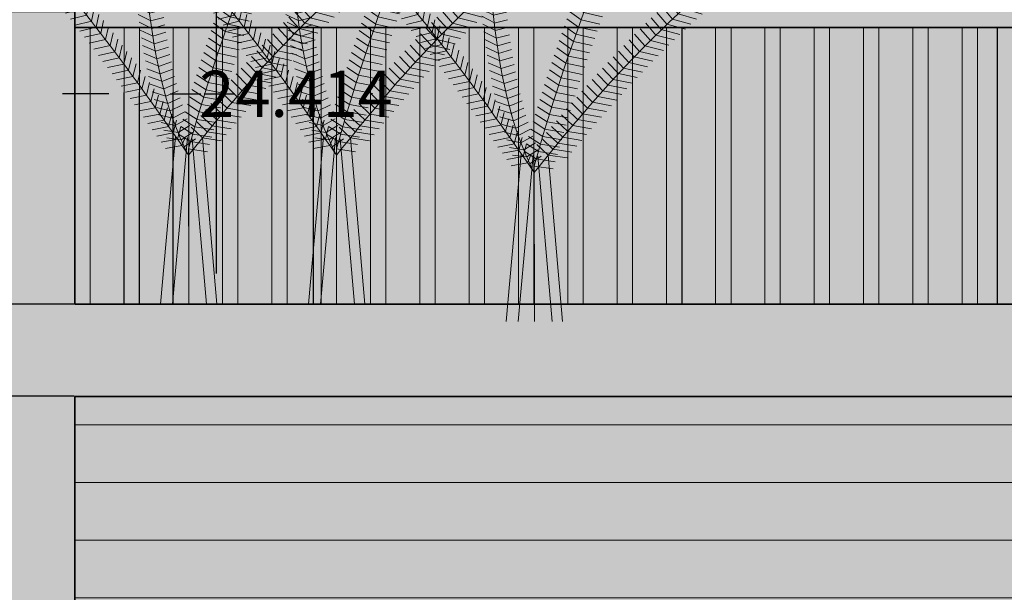
# Model space of a CAD drawing. Units: inches. Extents: x 184 to 649, y 215 to 818.
# Tile 5 of 9: x 254 to 382, y 473 to 548. Entities that reach past the tile are written whole.
import ezdxf

# ---------------------------------------------------------------- set-up
doc = ezdxf.new("R2010")
doc.units = ezdxf.units.IN
doc.header["$MEASUREMENT"] = 0
for name, color, linetype, lineweight in [('A-ANNO-DIMS', 2, 'Continuous', 18), ('A-DOOR', 4, 'Continuous', 25), ('A-ELEV', 7, 'Continuous', 35), ('A-ELEV-FILL', 9, 'Continuous', 13), ('A-ELEV-PATT', 8, 'Continuous', 13), ('A-ELEV-RAIL', 8, 'Continuous', 18), ('L-PLNT', 84, 'Continuous', 13)]:
    doc.layers.add(name, color=color, linetype=linetype, lineweight=lineweight)
doc.styles.get("Standard").update_dxf_attribs({"font": 'arial.ttf'})
doc.dimstyles.get("Standard").update_dxf_attribs({"dimtxt": 6, "dimasz": 4, "dimexe": 0.18, "dimexo": 0.0625, "dimgap": 0.09, "dimtad": 0, "dimtih": 1, "dimtoh": 1, "dimdec": 0, "dimzin": 0, "dimdsep": 46, "dimlunit": 3, "dimtxsty": 'Standard', "dimcen": 0.09, "dimadec": 0, "dimazin": 0, "dimtfac": 1, "dimtdec": 0, "dimtofl": 0, "dimtmove": 0, "dimatfit": 3, "dimfxl": 1, "dimtolj": 1, "dimtzin": 0, "dimarcsym": 0})

# ---------------------------------------------------------------- blocks, each defined once
blk = doc.blocks.new('PLANT-PALM')
for p, q in [((274.94, 416.06), (273.31, 416.97)), ((274.8, 417.06), (274.61, 417.16)), ((274.73, 417.05), (276.46, 417.47)), ((274.87, 416.06), (276.6, 416.47)), ((299.15, 415.59), (297.73, 416.77)), ((299.55, 416.5), (298.76, 417.16)), ((299.55, 416.5), (301.94, 415.78)), ((300.78, 417.16), (302.34, 416.68)), ((275.06, 415.07), (273.44, 415.99)), ((275, 415.07), (276.73, 415.46)), ((298.74, 414.67), (297.33, 415.85)), ((299.14, 415.59), (301.53, 414.87)), ((275.18, 414.08), (273.57, 415)), ((275.3, 413.08), (273.69, 414.02)), ((275.12, 414.07), (276.85, 414.46)), ((297.95, 412.84), (296.52, 414.01)), ((298.34, 413.75), (296.92, 414.93)), ((298.34, 413.75), (300.74, 413.04)), ((298.74, 414.67), (301.13, 413.96)), ((275.4, 412.09), (273.8, 413.03)), ((275.23, 413.08), (276.97, 413.45)), ((275.34, 412.09), (277.08, 412.45)), ((297.55, 411.92), (296.12, 413.09)), ((297.94, 412.84), (300.34, 412.13)), ((275.51, 411.09), (273.9, 412.04)), ((275.44, 411.09), (277.18, 411.45)), ((296.76, 410.08), (295.33, 411.24)), ((297.16, 411), (295.73, 412.16)), ((297.55, 411.92), (299.94, 411.22)), ((275.6, 410.1), (274, 411.05)), ((275.69, 409.1), (274.1, 410.06)), ((275.54, 410.1), (277.28, 410.45)), ((296.38, 409.16), (294.94, 410.32)), ((296.76, 410.08), (299.16, 409.39)), ((297.16, 411), (299.55, 410.3)), ((275.78, 408.11), (274.19, 409.06)), ((275.63, 409.1), (277.38, 409.45)), ((295.99, 408.23), (294.55, 409.39)), ((296.37, 409.16), (298.78, 408.47)), ((275.87, 407.11), (274.28, 408.07)), ((275.72, 408.1), (277.47, 408.45)), ((275.81, 407.11), (277.55, 407.44)), ((295.22, 406.39), (293.78, 407.54)), ((295.6, 407.31), (294.16, 408.46)), ((295.99, 408.24), (298.39, 407.56)), ((275.95, 406.11), (274.36, 407.08)), ((276.03, 405.12), (274.44, 406.08)), ((275.89, 406.11), (277.64, 406.45)), ((294.84, 405.46), (293.39, 406.61)), ((295.22, 406.39), (297.62, 405.72)), ((295.6, 407.31), (298.01, 406.64)), ((276.11, 404.12), (274.52, 405.08)), ((275.97, 405.11), (277.72, 405.45)), ((294.46, 404.54), (293.01, 405.68)), ((294.84, 405.46), (297.25, 404.8)), ((276.19, 403.12), (274.6, 404.09)), ((276.05, 404.12), (277.8, 404.45)), ((293.71, 402.68), (292.26, 403.82)), ((294.08, 403.61), (292.63, 404.75)), ((294.08, 403.61), (296.49, 402.96)), ((294.46, 404.54), (296.87, 403.88)), ((276.27, 402.13), (274.68, 403.09)), ((276.13, 403.12), (277.88, 403.45)), ((276.21, 402.12), (277.96, 402.46)), ((293.34, 401.76), (291.88, 402.89)), ((293.71, 402.68), (296.12, 402.04)), ((276.35, 401.13), (274.75, 402.09)), ((276.43, 400.13), (274.83, 401.09)), ((276.29, 401.13), (278.04, 401.46)), ((292.6, 399.9), (291.14, 401.02)), ((292.97, 400.83), (291.51, 401.95)), ((293.34, 401.76), (295.75, 401.12)), ((276.51, 399.14), (274.91, 400.09)), ((276.37, 400.13), (278.12, 400.47)), ((292.24, 398.97), (290.77, 400.08)), ((292.6, 399.9), (295.02, 399.27)), ((292.97, 400.83), (295.38, 400.2)), ((276.59, 398.14), (274.99, 399.09)), ((276.45, 399.13), (278.2, 399.47)), ((276.53, 398.14), (278.28, 398.48)), ((291.87, 398.03), (290.41, 399.15)), ((292.24, 398.97), (294.65, 398.35)), ((262.25, 396.34), (262.49, 398.02)), ((262.93, 395.6), (263.18, 397.28)), ((276.67, 397.14), (275.07, 398.09)), ((276.76, 396.15), (275.15, 397.08)), ((276.62, 397.14), (278.36, 397.49)), ((291.16, 396.17), (289.68, 397.27)), ((291.51, 397.1), (290.04, 398.21)), ((291.51, 397.1), (293.94, 396.5)), ((291.87, 398.03), (294.29, 397.42)), ((263.6, 394.85), (263.86, 396.53)), ((276.84, 395.15), (275.23, 396.08)), ((276.7, 396.14), (278.45, 396.5)), ((290.8, 395.23), (289.33, 396.34)), ((291.16, 396.17), (293.58, 395.57)), ((262.93, 395.59), (260.85, 394.94)), ((263.6, 394.85), (261.51, 394.21)), ((264.26, 394.11), (264.53, 395.78)), ((264.91, 393.35), (265.2, 395.02)), ((276.94, 394.16), (275.32, 395.08)), ((276.79, 395.15), (278.54, 395.51)), ((276.89, 394.15), (278.63, 394.52)), ((290.45, 394.3), (288.97, 395.4)), ((290.8, 395.23), (293.23, 394.64)), ((264.26, 394.1), (262.17, 393.48)), ((264.92, 393.35), (262.82, 392.74)), ((265.57, 392.59), (265.86, 394.26)), ((266.21, 391.83), (266.52, 393.5)), ((277.03, 393.16), (275.41, 394.07)), ((276.99, 393.16), (278.72, 393.54)), ((289.75, 392.42), (288.27, 393.51)), ((290.1, 393.36), (288.62, 394.45)), ((290.1, 393.36), (292.53, 392.78)), ((290.45, 394.3), (292.88, 393.71)), ((302.82, 391.73), (301.57, 393.3)), ((303.57, 392.39), (302.33, 393.98)), ((265.57, 392.59), (263.47, 391.99)), ((266.85, 391.06), (267.17, 392.73)), ((277.13, 392.17), (275.5, 393.07)), ((277.24, 391.17), (275.6, 392.06)), ((277.09, 392.16), (278.82, 392.55)), ((289.41, 391.48), (287.92, 392.57)), ((289.75, 392.42), (292.18, 391.85)), ((302.08, 391.06), (300.81, 392.62)), ((266.22, 391.82), (264.11, 391.25)), ((266.86, 391.06), (264.75, 390.49)), ((267.49, 390.29), (267.81, 391.95)), ((268.12, 389.51), (268.45, 391.17)), ((277.35, 390.18), (275.71, 391.05)), ((277.19, 391.17), (278.93, 391.57)), ((288.73, 389.6), (287.23, 390.68)), ((289.07, 390.54), (287.57, 391.62)), ((289.41, 391.48), (291.84, 390.92)), ((300.61, 389.7), (299.32, 391.25)), ((301.34, 390.38), (300.06, 391.94)), ((302.08, 391.06), (304.47, 390.35)), ((302.82, 391.73), (305.21, 391)), ((267.49, 390.29), (265.38, 389.73)), ((268.12, 389.51), (266.01, 388.97)), ((268.75, 388.73), (269.09, 390.39)), ((269.37, 387.95), (269.72, 389.61)), ((277.47, 389.19), (275.82, 390.05)), ((277.31, 390.18), (279.04, 390.59)), ((277.43, 389.18), (279.15, 389.61)), ((288.39, 388.66), (286.89, 389.73)), ((288.73, 389.6), (291.16, 389.05)), ((289.07, 390.54), (291.5, 389.98)), ((299.16, 388.32), (297.85, 389.85)), ((299.88, 389.01), (298.59, 390.55)), ((300.61, 389.7), (303.01, 389.03)), ((301.34, 390.38), (303.74, 389.69)), ((268.75, 388.73), (266.64, 388.2)), ((269.99, 387.16), (270.34, 388.82)), ((277.6, 388.2), (275.94, 389.04)), ((277.56, 388.19), (279.28, 388.63)), ((288.06, 387.72), (286.56, 388.79)), ((288.39, 388.66), (290.83, 388.12)), ((297.74, 386.91), (296.41, 388.42)), ((298.45, 387.62), (297.13, 389.14)), ((299.16, 388.32), (301.58, 387.68)), ((299.88, 389.01), (302.29, 388.36)), ((269.37, 387.95), (267.26, 387.43)), ((269.99, 387.16), (267.87, 386.65)), ((270.6, 386.37), (270.97, 388.03)), ((271.21, 385.58), (271.58, 387.24)), ((277.73, 387.21), (276.06, 388.03)), ((277.87, 386.22), (276.2, 387.03)), ((277.69, 387.2), (279.41, 387.66)), ((287.4, 385.83), (285.89, 386.89)), ((287.73, 386.77), (286.22, 387.84)), ((288.06, 387.72), (290.5, 387.18)), ((296.33, 385.49), (294.99, 386.98)), ((297.03, 386.2), (295.69, 387.71)), ((297.74, 386.91), (300.16, 386.31)), ((298.45, 387.62), (300.87, 387)), ((270.61, 386.37), (268.48, 385.87)), ((271.22, 385.58), (269.09, 385.09)), ((271.82, 384.79), (272.2, 386.44)), ((272.42, 383.99), (272.8, 385.64)), ((278.02, 385.23), (276.34, 386.02)), ((277.83, 386.21), (279.55, 386.69)), ((277.99, 385.22), (279.69, 385.72)), ((287.08, 384.88), (285.56, 385.94)), ((287.4, 385.83), (289.84, 385.31)), ((287.73, 386.77), (290.17, 386.25)), ((295.64, 384.77), (294.28, 386.26)), ((297.03, 386.2), (299.46, 385.61)), ((271.82, 384.79), (269.7, 384.3)), ((273.02, 383.19), (273.41, 384.84)), ((278.18, 384.24), (276.49, 385.01)), ((278.15, 384.24), (279.85, 384.75)), ((286.76, 383.94), (285.24, 384.98)), ((287.08, 384.88), (289.52, 384.37)), ((294.26, 383.32), (292.89, 384.79)), ((294.95, 384.05), (293.58, 385.53)), ((295.64, 384.77), (298.07, 384.21)), ((296.33, 385.49), (298.76, 384.92)), ((272.43, 383.99), (270.3, 383.51)), ((273.03, 383.19), (270.9, 382.72)), ((273.62, 382.39), (274.01, 384.04)), ((274.21, 381.58), (274.61, 383.23)), ((278.36, 383.26), (276.65, 384)), ((278.54, 382.28), (276.83, 382.99)), ((278.32, 383.25), (280.02, 383.79)), ((286.12, 382.04), (284.6, 383.08)), ((286.44, 382.99), (284.92, 384.03)), ((286.75, 383.94), (289.2, 383.43)), ((292.9, 381.85), (291.51, 383.31)), ((293.58, 382.59), (292.2, 384.05)), ((294.26, 383.32), (296.7, 382.79)), ((294.95, 384.05), (297.38, 383.5)), ((273.62, 382.39), (271.49, 381.93)), ((274.8, 380.78), (275.21, 382.42)), ((278.74, 381.3), (277.01, 381.99)), ((278.51, 382.27), (280.2, 382.83)), ((278.71, 381.29), (280.39, 381.87)), ((285.81, 381.09), (284.28, 382.12)), ((286.12, 382.04), (288.57, 381.55)), ((286.44, 382.99), (288.88, 382.49)), ((291.56, 380.37), (290.15, 381.81)), ((292.23, 381.11), (290.83, 382.56)), ((292.9, 381.85), (295.35, 381.35)), ((293.58, 382.59), (296.02, 382.07)), ((274.22, 381.58), (272.09, 381.13)), ((274.81, 380.78), (272.68, 380.33)), ((275.39, 379.97), (275.8, 381.61)), ((275.98, 379.16), (276.39, 380.8)), ((278.95, 380.32), (277.21, 380.98)), ((278.92, 380.31), (280.59, 380.92)), ((285.5, 380.14), (283.97, 381.16)), ((285.81, 381.09), (288.26, 380.61)), ((290.9, 379.63), (289.48, 381.06)), ((292.23, 381.11), (294.68, 380.62)), ((275.4, 379.97), (273.26, 379.53)), ((275.99, 379.16), (273.85, 378.72)), ((276.56, 378.35), (276.98, 379.99)), ((277.14, 377.53), (277.56, 379.18)), ((279.17, 379.35), (277.42, 379.97)), ((279.15, 379.34), (280.81, 379.98)), ((284.9, 378.23), (283.36, 379.24)), ((285.2, 379.18), (283.66, 380.2)), ((285.2, 379.18), (287.65, 378.72)), ((285.5, 380.14), (287.95, 379.67)), ((289.58, 378.12), (288.15, 379.54)), ((290.23, 378.87), (288.81, 380.3)), ((290.9, 379.63), (293.35, 379.16)), ((291.56, 380.37), (294.01, 379.89)), ((276.57, 378.35), (274.43, 377.92)), ((279.41, 378.38), (277.65, 378.97)), ((277.72, 376.72), (278.15, 378.36)), ((279.67, 377.41), (277.9, 377.96)), ((279.39, 378.37), (281.04, 379.04)), ((279.65, 377.4), (281.29, 378.11)), ((284.6, 377.27), (283.06, 378.28)), ((284.9, 378.23), (287.35, 377.78)), ((288.27, 376.61), (286.83, 378.01)), ((288.92, 377.36), (287.49, 378.78)), ((289.58, 378.12), (292.03, 377.67)), ((290.23, 378.87), (292.69, 378.42)), ((277.15, 377.53), (275.02, 377.11)), ((277.74, 376.72), (275.6, 376.3)), ((279.95, 376.45), (278.16, 376.96)), ((278.3, 375.9), (278.73, 377.55)), ((278.88, 375.09), (279.31, 376.73)), ((279.93, 376.44), (281.55, 377.18)), ((284.31, 376.32), (282.76, 377.32)), ((284.6, 377.28), (287.06, 376.83)), ((287.63, 375.84), (286.18, 377.24)), ((288.27, 376.61), (290.73, 376.18)), ((288.92, 377.36), (291.38, 376.93)), ((278.31, 375.91), (276.18, 375.49)), ((280.24, 375.49), (278.44, 375.96)), ((279.46, 374.27), (279.88, 375.91)), ((280.23, 375.49), (281.83, 376.27)), ((280.55, 374.54), (282.13, 375.36)), ((283.73, 374.4), (282.18, 375.39)), ((284.02, 375.36), (282.47, 376.36)), ((284.02, 375.36), (286.48, 374.94)), ((284.31, 376.32), (286.77, 375.89)), ((286.34, 374.31), (284.89, 375.7)), ((286.98, 375.08), (285.53, 376.47)), ((287.63, 375.84), (290.09, 375.43)), ((278.89, 375.09), (276.75, 374.67)), ((279.47, 374.27), (277.33, 373.86)), ((280.56, 374.55), (278.75, 374.97)), ((280.03, 373.45), (280.46, 375.09)), ((280.61, 372.64), (281.04, 374.28)), ((280.89, 373.6), (282.45, 374.46)), ((283.45, 373.44), (281.89, 374.43)), ((285.07, 372.76), (283.61, 374.14)), ((283.73, 374.4), (286.2, 373.99)), ((285.71, 373.54), (284.24, 374.92)), ((286.34, 374.31), (288.81, 373.91)), ((286.98, 375.08), (289.45, 374.67)), ((280.05, 373.46), (277.91, 373.04)), ((280.9, 373.61), (279.08, 373.97)), ((281.26, 372.67), (279.43, 372.98)), ((281.18, 371.82), (281.61, 373.46)), ((281.26, 372.67), (282.79, 373.58)), ((283.18, 372.48), (281.61, 373.46)), ((284.44, 371.99), (282.97, 373.36)), ((283.45, 373.44), (285.92, 373.04)), ((285.07, 372.76), (287.54, 372.39)), ((285.71, 373.54), (288.17, 373.15)), ((280.62, 372.64), (278.48, 372.23)), ((281.2, 371.82), (279.05, 371.41)), ((281.65, 371.75), (279.81, 372)), ((282.9, 371.52), (281.33, 372.49)), ((281.65, 371.75), (283.15, 372.7)), ((281.77, 371), (282.24, 372.12)), ((282.07, 370.84), (283.54, 371.85)), ((282.9, 371.52), (285.37, 371.14)), ((283.18, 372.48), (285.64, 372.09)), ((284.44, 371.99), (286.91, 371.62)), ((281.77, 371), (279.63, 370.59)), ((282.63, 370.56), (285.1, 370.19))]:
    blk.add_line(p, q)
blk.add_open_spline([(274.68, 417.16), (274.77, 416.57), (276.95, 400.47), (276.36, 381.5), (282.64, 369.73)], degree=3, knots=[87.299959, 87.299959, 87.299959, 87.299959, 88.780677, 127.704389, 127.704389, 127.704389, 127.704389])
for points in [[(282.63, 370.56), (286.61, 384.99), (292.84, 401.43), (299.95, 417.41)], [(282.55, 369.88), (275.93, 379.33), (269.31, 388.78), (261.65, 396.98)], [(282.64, 369.73), (290.67, 379.89), (297.61, 387.15), (303.65, 392.43)]]:
    blk.add_open_spline(points, degree=3)
blk = doc.blocks.new('PLANT-STEM')
for p, q in [((319.07, 530.29), (317.11, 508.48)), ((320.61, 530.15), (318.67, 508.48)), ((321.21, 529.98), (323.08, 508.48)), ((322.56, 530.1), (324.44, 508.48)), ((320.76, 528.67), (320.77, 508.48))]:
    blk.add_line(p, q)
blk = doc.blocks.new('DOOR-BALCONY')
for points in [[(340, 548.73), (340, 594.73), (292, 594.73), (292, 548.73)], [(336, 578.73), (336, 590.73), (296, 590.73), (296, 578.73)], [(296, 574.73), (296, 548.73)], [(336, 548.73), (336, 574.73)], [(292, 546.73), (292, 510.73), (340, 510.73), (340, 546.73)]]:
    blk.add_lwpolyline(points)
blk = doc.blocks.new('*D7')
at = {"layer": 'A-ANNO-DIMS', "color": 0, "lineweight": -2, "transparency": 16777216}
for p, q in [((291.94, 594.73), (279.22, 594.73)), ((279.4, 590.73), (279.4, 555.92)), ((279.4, 514.73), (279.4, 549.53)), ((291.94, 510.73), (279.22, 510.73))]:
    blk.add_line(p, q, dxfattribs=at)
at = {"layer": 'A-ANNO-DIMS', "color": 0, "transparency": 16777216}
for points in [[(278.73, 590.73), (280.07, 590.73), (279.4, 594.73)], [(278.73, 514.73), (280.07, 514.73), (279.4, 510.73)]]:
    blk.add_solid(points, dxfattribs=at)
at = {"layer": 'Defpoints', "color": 0, "transparency": 16777216}
for p in [(279.4, 594.73), (292, 594.73), (292, 510.73)]:
    blk.add_point(p, dxfattribs=at)
at = {"layer": 'A-ANNO-DIMS', "color": 0, "transparency": 16777216, "insert": (279.4, 552.73), "char_height": 6, "attachment_point": 5}
blk.add_mtext('\\A1;BALCONY DOOR 84 TYP.', dxfattribs=at)
blk = doc.blocks.new('*D35')
at = {"layer": 'A-ANNO-DIMS', "color": 0, "lineweight": -2, "transparency": 16777216}
for p, q in [((260.91, 498.73), (196.12, 498.73)), ((196.3, 494.73), (196.3, 437.38)), ((196.3, 373.73), (196.3, 431.07)), ((260.91, 369.73), (196.12, 369.73))]:
    blk.add_line(p, q, dxfattribs=at)
at = {"layer": 'A-ANNO-DIMS', "color": 0, "transparency": 16777216}
for points in [[(195.63, 494.73), (196.96, 494.73), (196.3, 498.73)], [(195.63, 373.73), (196.96, 373.73), (196.3, 369.73)]]:
    blk.add_solid(points, dxfattribs=at)
at = {"layer": 'Defpoints', "color": 0, "transparency": 16777216}
for p in [(196.3, 498.73), (260.97, 498.73), (260.97, 369.73)]:
    blk.add_point(p, dxfattribs=at)
at = {"layer": 'A-ANNO-DIMS', "color": 0, "transparency": 16777216, "insert": (196.3, 434.23), "char_height": 6, "attachment_point": 5}
blk.add_mtext('\\A1;129', dxfattribs=at)
blk = doc.blocks.new('*D36')
at = {"layer": 'A-ANNO-DIMS', "color": 0, "lineweight": -2, "transparency": 16777216}
for p, q in [((196.3, 510.73), (196.3, 514.73)), ((196.3, 514.73), (200.3, 514.73)), ((260.91, 510.73), (196.12, 510.73)), ((196.3, 502.73), (196.3, 506.73)), ((260.91, 498.73), (196.12, 498.73))]:
    blk.add_line(p, q, dxfattribs=at)
at = {"layer": 'A-ANNO-DIMS', "color": 0, "transparency": 16777216}
for points in [[(195.63, 506.73), (196.96, 506.73), (196.3, 510.73)], [(195.63, 502.73), (196.96, 502.73), (196.3, 498.73)]]:
    blk.add_solid(points, dxfattribs=at)
at = {"layer": 'Defpoints', "color": 0, "transparency": 16777216}
for p in [(196.3, 510.73), (260.97, 510.73), (260.97, 498.73)]:
    blk.add_point(p, dxfattribs=at)
at = {"layer": 'A-ANNO-DIMS', "color": 0, "transparency": 16777216, "insert": (204.37, 514.73), "char_height": 6, "attachment_point": 5}
blk.add_mtext('\\A1;12', dxfattribs=at)
blk = doc.blocks.new('*D37')
at = {"layer": 'A-ANNO-DIMS', "color": 0, "lineweight": -2, "transparency": 16777216}
for p, q in [((260.91, 548.73), (196.12, 548.73)), ((196.3, 544.73), (196.3, 532.88)), ((196.3, 514.73), (196.3, 526.57)), ((260.91, 510.73), (196.12, 510.73))]:
    blk.add_line(p, q, dxfattribs=at)
at = {"layer": 'A-ANNO-DIMS', "color": 0, "transparency": 16777216}
for points in [[(195.63, 544.73), (196.96, 544.73), (196.3, 548.73)], [(195.63, 514.73), (196.96, 514.73), (196.3, 510.73)]]:
    blk.add_solid(points, dxfattribs=at)
at = {"layer": 'Defpoints', "color": 0, "transparency": 16777216}
for p in [(196.3, 548.73), (260.97, 548.73), (260.97, 510.73)]:
    blk.add_point(p, dxfattribs=at)
at = {"layer": 'A-ANNO-DIMS', "color": 0, "transparency": 16777216, "insert": (196.3, 529.73), "char_height": 6, "attachment_point": 5}
blk.add_mtext('\\A1;38', dxfattribs=at)
blk = doc.blocks.new('*D57')
at = {"layer": 'A-ANNO-DIMS', "color": 0, "lineweight": -2, "transparency": 16777216}
for p, q in [((263.39, 538.08), (259.39, 538.08)), ((267.39, 510.79), (267.39, 538.26)), ((269.39, 510.79), (269.39, 538.26)), ((273.39, 538.08), (277.39, 538.08))]:
    blk.add_line(p, q, dxfattribs=at)
at = {"layer": 'A-ANNO-DIMS', "color": 0, "transparency": 16777216}
for points in [[(263.39, 538.74), (263.39, 537.41), (267.39, 538.08)], [(273.39, 538.74), (273.39, 537.41), (269.39, 538.08)]]:
    blk.add_solid(points, dxfattribs=at)
at = {"layer": 'Defpoints', "color": 0, "transparency": 16777216}
for p in [(269.39, 538.08), (267.39, 510.73), (269.39, 510.73)]:
    blk.add_point(p, dxfattribs=at)
at = {"layer": 'A-ANNO-DIMS', "color": 0, "transparency": 16777216, "insert": (279.46, 538.08), "char_height": 6, "attachment_point": 5}
blk.add_mtext('\\A1;2', dxfattribs=at)
blk = doc.blocks.new('*D58')
at = {"layer": 'A-ANNO-DIMS', "color": 0, "lineweight": -2, "transparency": 16777216}
for p, q in [((265.39, 538.08), (261.39, 538.08)), ((269.39, 510.79), (269.39, 538.26)), ((273.8, 510.79), (273.8, 538.26)), ((277.8, 538.08), (281.8, 538.08))]:
    blk.add_line(p, q, dxfattribs=at)
at = {"layer": 'A-ANNO-DIMS', "color": 0, "transparency": 16777216}
for points in [[(265.39, 538.74), (265.39, 537.41), (269.39, 538.08)], [(277.8, 538.74), (277.8, 537.41), (273.8, 538.08)]]:
    blk.add_solid(points, dxfattribs=at)
at = {"layer": 'Defpoints', "color": 0, "transparency": 16777216}
for p in [(273.8, 538.08), (269.39, 510.73), (273.8, 510.73)]:
    blk.add_point(p, dxfattribs=at)
at = {"layer": 'A-ANNO-DIMS', "color": 0, "transparency": 16777216, "insert": (292.12, 538.08), "char_height": 6, "attachment_point": 5}
blk.add_mtext('\\A1;4.414', dxfattribs=at)

msp = doc.modelspace()

# ---------------------------------------------------------------- hatches: boundary and pattern name
at = {"layer": 'A-ELEV-FILL'}
h = msp.add_hatch(color=256, dxfattribs=at)
h.dxf.hatch_style = 1
h.paths.add_polyline_path([(452.9726, 369.7265), (248.9726, 369.7265), (248.9726, 246.7265), (275.9726, 246.7265), (275.9726, 328.7265), (437.9726, 328.7265), (437.9726, 246.7265), (446.6666, 246.7265), (452.9726, 282.7265)])
h.paths.add_polyline_path([(275.9726, 340.7265), (275.9726, 354.7265), (437.9726, 354.7265), (437.9726, 340.7265)], flags=16)
h.paths.add_polyline_path([(452.9726, 510.7265), (260.9726, 510.7265), (260.9726, 642.7265), (260.9726, 699.7265), (367.0226, 699.7265), (373.9381, 706.7265), (260.9726, 706.7265), (260.9726, 715.7265), (382.8295, 715.7265), (389.745, 722.7265), (260.9726, 722.7265), (260.9726, 731.7265), (398.6364, 731.7265), (405.5519, 738.7265), (260.9726, 738.7265), (260.9726, 747.7265), (414.4433, 747.7265), (421.3588, 754.7265), (260.9726, 754.7265), (260.9726, 763.7265), (430.2502, 763.7265), (437.1657, 770.7265), (260.9726, 770.7265), (260.9726, 779.7265), (446.057, 779.7265), (452.9726, 786.7265), (248.9726, 786.7265), (248.9726, 369.7265), (260.9726, 369.7265), (260.9726, 498.7265), (452.9726, 498.7265)])
h = msp.add_hatch(color=256, dxfattribs=at)
h.dxf.hatch_style = 1
h.paths.add_polyline_path([(380.9726, 453.5037), (422.2268, 453.5037), (422.2268, 474.7265), (260.9726, 474.7265), (260.9726, 369.7265), (291.9998, 369.7265), (291.9998, 453.5037), (339.9998, 453.5037), (339.9998, 369.7265), (380.9726, 369.7265)])
h.paths.add_polyline_path([(437.9726, 328.7265), (275.9726, 328.7265), (275.9726, 246.7265), (437.9726, 246.7265)])
h.paths.add_polyline_path([(581.9726, 759.7265), (521.9726, 759.7265), (521.9726, 441.2233), (581.9726, 441.2233)])
h.paths.add_polyline_path([(560.9726, 582.4749), (560.9726, 477.2233), (542.9726, 477.2233), (542.9726, 582.4749)], flags=16)
h.paths.add_polyline_path([(560.9726, 618.4749), (542.9726, 618.4749), (542.9726, 723.7265), (560.9726, 723.7265)], flags=16)
h = msp.add_hatch(color=256, dxfattribs=at)
h.dxf.hatch_style = 1
h.paths.add_polyline_path([(452.9726, 548.7265), (260.9726, 548.7265), (260.9726, 546.7265), (452.9726, 546.7265)])
h.paths.add_polyline_path([(262.9726, 546.7265), (260.9726, 546.7265), (260.9726, 510.7265), (262.9726, 510.7265)])
h.paths.add_polyline_path([(269.3864, 546.7265), (267.3864, 546.7265), (267.3864, 510.7265), (269.3864, 510.7265)])
h.paths.add_polyline_path([(275.8001, 546.7265), (273.8001, 546.7265), (273.8001, 510.7265), (275.8001, 510.7265)])
h.paths.add_polyline_path([(282.2139, 546.7265), (280.2139, 546.7265), (280.2139, 510.7265), (282.2139, 510.7265)])
h.paths.add_polyline_path([(288.6277, 546.7265), (286.6277, 546.7265), (286.6277, 510.7265), (288.6277, 510.7265)])
h.paths.add_polyline_path([(295.0415, 546.7265), (293.0415, 546.7265), (293.0415, 510.7265), (295.0415, 510.7265)])
h.paths.add_polyline_path([(301.4553, 546.7265), (299.4553, 546.7265), (299.4553, 514.7265), (301.4553, 514.7265)])
h.paths.add_polyline_path([(307.8691, 546.7265), (305.8691, 546.7265), (305.8691, 514.7265), (307.8691, 514.7265)])
h.paths.add_polyline_path([(314.2829, 546.7265), (312.2829, 546.7265), (312.2829, 514.7265), (314.2829, 514.7265)])
h.paths.add_polyline_path([(320.6967, 546.7265), (318.6967, 546.7265), (318.6967, 514.7265), (320.6967, 514.7265)])
h.paths.add_polyline_path([(327.1105, 546.7265), (325.1105, 546.7265), (325.1105, 514.7265), (327.1105, 514.7265)])
h.paths.add_polyline_path([(333.5243, 546.7265), (331.5243, 546.7265), (331.5243, 514.7265), (333.5243, 514.7265)])
h.paths.add_polyline_path([(339.9381, 546.7265), (337.9381, 546.7265), (337.9381, 510.7265), (339.9381, 510.7265)])
h.paths.add_polyline_path([(346.3519, 546.7265), (344.3519, 546.7265), (344.3519, 510.7265), (346.3519, 510.7265)])
h.paths.add_polyline_path([(352.7657, 546.7265), (350.7657, 546.7265), (350.7657, 510.7265), (352.7657, 510.7265)])
h.paths.add_polyline_path([(359.1795, 546.7265), (357.1795, 546.7265), (357.1795, 510.7265), (359.1795, 510.7265)])
h.paths.add_polyline_path([(365.5932, 546.7265), (363.5932, 546.7265), (363.5932, 510.7265), (365.5932, 510.7265)])
h.paths.add_polyline_path([(372.007, 546.7265), (370.007, 546.7265), (370.007, 510.7265), (372.007, 510.7265)])
h.paths.add_polyline_path([(378.4208, 546.7265), (376.4208, 546.7265), (376.4208, 510.7265), (378.4208, 510.7265)])
h.paths.add_polyline_path([(384.8346, 546.7265), (382.8346, 546.7265), (382.8346, 510.7265), (384.8346, 510.7265)])
h.paths.add_polyline_path([(391.2484, 546.7265), (389.2484, 546.7265), (389.2484, 514.7265), (391.2484, 514.7265)])
h.paths.add_polyline_path([(397.6622, 546.7265), (395.6622, 546.7265), (395.6622, 514.7265), (397.6622, 514.7265)])
h.paths.add_polyline_path([(404.076, 546.7265), (402.076, 546.7265), (402.076, 514.7265), (404.076, 514.7265)])
h.paths.add_polyline_path([(410.4898, 546.7265), (408.4898, 546.7265), (408.4898, 514.7265), (410.4898, 514.7265)])
h.paths.add_polyline_path([(416.9036, 546.7265), (414.9036, 546.7265), (414.9036, 514.7265), (416.9036, 514.7265)])
h.paths.add_polyline_path([(423.3174, 546.7265), (421.3174, 546.7265), (421.3174, 514.7265), (423.3174, 514.7265)])
h.paths.add_polyline_path([(423.3174, 514.7265), (421.3174, 514.7265), (421.3174, 510.7265), (423.3174, 510.7265)])
h.paths.add_polyline_path([(416.9036, 514.7265), (414.9036, 514.7265), (414.9036, 510.7265), (416.9036, 510.7265)])
h.paths.add_polyline_path([(410.4898, 514.7265), (408.4898, 514.7265), (408.4898, 510.7265), (410.4898, 510.7265)])
h.paths.add_polyline_path([(404.076, 514.7265), (402.076, 514.7265), (402.076, 510.7265), (404.076, 510.7265)])
h.paths.add_polyline_path([(397.6622, 514.7265), (395.6622, 514.7265), (395.6622, 510.7265), (397.6622, 510.7265)])
h.paths.add_polyline_path([(391.2484, 514.7265), (389.2484, 514.7265), (389.2484, 510.7265), (391.2484, 510.7265)])
h.paths.add_polyline_path([(448.9726, 546.7265), (446.9726, 546.7265), (446.9726, 510.7265), (448.9726, 510.7265)])
h.paths.add_polyline_path([(442.5588, 546.7265), (440.5588, 546.7265), (440.5588, 510.7265), (442.5588, 510.7265)])
h.paths.add_polyline_path([(436.145, 546.7265), (434.145, 546.7265), (434.145, 510.7265), (436.145, 510.7265)])
h.paths.add_polyline_path([(429.7312, 546.7265), (428.9726, 546.7265), (428.9726, 510.7265), (429.7312, 510.7265)])
h.paths.add_polyline_path([(301.4553, 514.7265), (299.4553, 514.7265), (299.4553, 510.7265), (301.4553, 510.7265)])
h.paths.add_polyline_path([(307.8691, 514.7265), (305.8691, 514.7265), (305.8691, 510.7265), (307.8691, 510.7265)])
h.paths.add_polyline_path([(314.2829, 514.7265), (312.2829, 514.7265), (312.2829, 510.7265), (314.2829, 510.7265)])
h.paths.add_polyline_path([(320.6967, 514.7265), (318.6967, 514.7265), (318.6967, 510.7265), (320.6967, 510.7265)])
h.paths.add_polyline_path([(327.1105, 514.7265), (325.1105, 514.7265), (325.1105, 510.7265), (327.1105, 510.7265)])
h.paths.add_polyline_path([(333.5243, 514.7265), (331.5243, 514.7265), (331.5243, 510.7265), (333.5243, 510.7265)])
h = msp.add_hatch(color=256, dxfattribs=at)
h.dxf.hatch_style = 1
h.paths.add_polyline_path([(380.9726, 546.7265), (378.4208, 546.7265), (378.4208, 510.7265), (380.9726, 510.7265)])
h.paths.add_polyline_path([(376.4208, 546.7265), (372.007, 546.7265), (372.007, 510.7265), (376.4208, 510.7265)])
h.paths.add_polyline_path([(370.007, 546.7265), (365.5932, 546.7265), (365.5932, 510.7265), (370.007, 510.7265)])
h.paths.add_polyline_path([(363.5932, 546.7265), (359.1795, 546.7265), (359.1795, 510.7265), (363.5932, 510.7265)])
h.paths.add_polyline_path([(357.1795, 546.7265), (352.7657, 546.7265), (352.7657, 510.7265), (357.1795, 510.7265)])
h.paths.add_polyline_path([(350.7657, 546.7265), (346.3519, 546.7265), (346.3519, 510.7265), (350.7657, 510.7265)])
h.paths.add_polyline_path([(344.3519, 546.7265), (339.9998, 546.7265), (339.9998, 510.7265), (344.3519, 510.7265)])
h.paths.add_polyline_path([(267.3864, 546.7265), (262.9726, 546.7265), (262.9726, 510.7265), (267.3864, 510.7265)])
h.paths.add_polyline_path([(273.8001, 546.7265), (269.3864, 546.7265), (269.3864, 510.7265), (273.8001, 510.7265)])
h.paths.add_polyline_path([(280.2139, 546.7265), (275.8001, 546.7265), (275.8001, 510.7265), (280.2139, 510.7265)])
h.paths.add_polyline_path([(286.6277, 546.7265), (282.2139, 546.7265), (282.2139, 510.7265), (286.6277, 510.7265)])
h.paths.add_polyline_path([(291.9998, 546.7265), (288.6277, 546.7265), (288.6277, 510.7265), (291.9998, 510.7265)])
h = msp.add_hatch(color=256, dxfattribs=at)
h.dxf.hatch_style = 1
h.paths.add_polyline_path([(382.8346, 546.7265), (380.9726, 546.7265), (380.9726, 510.7265), (382.8346, 510.7265)])
h.paths.add_polyline_path([(421.3174, 514.7265), (416.9036, 514.7265), (416.9036, 510.7265), (421.3174, 510.7265)])
h.paths.add_polyline_path([(414.9036, 514.7265), (410.4898, 514.7265), (410.4898, 510.7265), (414.9036, 510.7265)])
h.paths.add_polyline_path([(408.4898, 514.7265), (404.076, 514.7265), (404.076, 510.7265), (408.4898, 510.7265)])
h.paths.add_polyline_path([(402.076, 514.7265), (397.6622, 514.7265), (397.6622, 510.7265), (402.076, 510.7265)])
h.paths.add_polyline_path([(395.6622, 514.7265), (391.2484, 514.7265), (391.2484, 510.7265), (395.6622, 510.7265)])
h.paths.add_polyline_path([(389.2484, 514.7265), (384.9726, 514.7265), (384.9726, 546.7265), (384.8346, 546.7265), (384.8346, 510.7265), (389.2484, 510.7265)])
h.paths.add_polyline_path([(293.0415, 546.7265), (291.9998, 546.7265), (291.9998, 510.7265), (293.0415, 510.7265)], flags=16)
h.paths.add_polyline_path([(299.4553, 514.7265), (295.9998, 514.7265), (295.9998, 546.7265), (295.0415, 546.7265), (295.0415, 510.7265), (299.4553, 510.7265)], flags=16)
h.paths.add_polyline_path([(337.9381, 546.7265), (335.9998, 546.7265), (335.9998, 514.7265), (333.5243, 514.7265), (333.5243, 510.7265), (337.9381, 510.7265)], flags=17)
h.paths.add_polyline_path([(339.9998, 546.7265), (339.9381, 546.7265), (339.9381, 510.7265), (339.9998, 510.7265)])
h = msp.add_hatch(color=256, dxfattribs=at)
h.dxf.hatch_style = 1
h.paths.add_polyline_path([(417.6041, 354.7265), (411.9199, 354.7265), (411.9199, 340.7265), (417.6041, 340.7265)])
h.paths.add_polyline_path([(409.9199, 354.7265), (404.2357, 354.7265), (404.2357, 340.7265), (409.9199, 340.7265)])
h.paths.add_polyline_path([(402.2357, 354.7265), (396.5515, 354.7265), (396.5515, 340.7265), (402.2357, 340.7265)])
h.paths.add_polyline_path([(394.5515, 354.7265), (388.8673, 354.7265), (388.8673, 340.7265), (394.5515, 340.7265)])
h.paths.add_polyline_path([(333.0778, 354.7265), (327.3936, 354.7265), (327.3936, 340.7265), (333.0778, 340.7265)])
h.paths.add_polyline_path([(325.3936, 354.7265), (319.7094, 354.7265), (319.7094, 340.7265), (325.3936, 340.7265)])
h.paths.add_polyline_path([(317.7094, 354.7265), (312.0252, 354.7265), (312.0252, 340.7265), (317.7094, 340.7265)])
h.paths.add_polyline_path([(310.0252, 354.7265), (304.341, 354.7265), (304.341, 340.7265), (310.0252, 340.7265)])
h.paths.add_polyline_path([(302.341, 354.7265), (296.6568, 354.7265), (296.6568, 340.7265), (302.341, 340.7265)])
h.paths.add_polyline_path([(421.3174, 546.7265), (416.9036, 546.7265), (416.9036, 514.7265), (421.3174, 514.7265)])
h.paths.add_polyline_path([(414.9036, 546.7265), (410.4898, 546.7265), (410.4898, 514.7265), (414.9036, 514.7265)])
h.paths.add_polyline_path([(402.076, 546.7265), (397.6622, 546.7265), (397.6622, 514.7265), (402.076, 514.7265)])
h.paths.add_polyline_path([(395.6622, 546.7265), (391.2484, 546.7265), (391.2484, 514.7265), (395.6622, 514.7265)])
h.paths.add_polyline_path([(389.2484, 546.7265), (384.9726, 546.7265), (384.9726, 514.7265), (389.2484, 514.7265)])
h.paths.add_polyline_path([(408.4898, 546.7265), (404.076, 546.7265), (404.076, 514.7265), (408.4898, 514.7265)])
h.paths.add_polyline_path([(335.9998, 546.7265), (333.5243, 546.7265), (333.5243, 514.7265), (335.9998, 514.7265)])
h.paths.add_polyline_path([(331.5243, 546.7265), (327.1105, 546.7265), (327.1105, 514.7265), (331.5243, 514.7265)])
h.paths.add_polyline_path([(325.1105, 546.7265), (320.6967, 546.7265), (320.6967, 514.7265), (325.1105, 514.7265)])
h.paths.add_polyline_path([(318.6967, 546.7265), (314.2829, 546.7265), (314.2829, 514.7265), (318.6967, 514.7265)])
h.paths.add_polyline_path([(312.2829, 546.7265), (307.8691, 546.7265), (307.8691, 514.7265), (312.2829, 514.7265)])
h.paths.add_polyline_path([(305.8691, 546.7265), (301.4553, 546.7265), (301.4553, 514.7265), (305.8691, 514.7265)])
h.paths.add_polyline_path([(299.4553, 546.7265), (295.9998, 546.7265), (295.9998, 514.7265), (299.4553, 514.7265)])
h = msp.add_hatch(color=256, dxfattribs=at)
h.dxf.hatch_style = 1
h.paths.add_polyline_path([(305.8691, 514.7265), (301.4553, 514.7265), (301.4553, 510.7265), (305.8691, 510.7265)])
h.paths.add_polyline_path([(312.2829, 514.7265), (307.8691, 514.7265), (307.8691, 510.7265), (312.2829, 510.7265)])
h.paths.add_polyline_path([(318.6967, 514.7265), (314.2829, 514.7265), (314.2829, 510.7265), (318.6967, 510.7265)])
h.paths.add_polyline_path([(325.1105, 514.7265), (320.6967, 514.7265), (320.6967, 510.7265), (325.1105, 510.7265)])
h.paths.add_polyline_path([(331.5243, 514.7265), (327.1105, 514.7265), (327.1105, 510.7265), (331.5243, 510.7265)])
h = msp.add_hatch(color=256, dxfattribs=at)
h.dxf.hatch_style = 1
h.paths.add_polyline_path([(437.9726, 498.7265), (260.9726, 498.7265), (260.9726, 474.7265), (422.2268, 474.7265), (422.2268, 453.5037), (428.9726, 453.5037), (428.9726, 417.0753), (445.4726, 417.0753), (445.4726, 437.9607), (437.9726, 437.9607)])
at = {"layer": 'A-ELEV-PATT'}
h = msp.add_hatch(dxfattribs=at)
h.set_pattern_fill('ANSI31', color=256, scale=60, angle=135)
h.paths.add_polyline_path([(437.9726, 498.7265), (260.9726, 498.7265), (260.9726, 369.7265), (291.9998, 369.7265), (291.9998, 453.5037), (339.9998, 453.5037), (339.9998, 369.7265), (380.9726, 369.7265), (380.9726, 453.5037), (428.9726, 453.5037), (428.9726, 417.0753), (445.4726, 417.0753), (445.4726, 437.9607), (437.9726, 437.9607)])

# ---------------------------------------------------------------- linework, layer by layer
at = {"layer": 'A-ELEV'}
for p, q in [((260.9726, 642.7265), (260.9726, 510.7265)), ((452.9726, 546.7265), (260.9726, 546.7265)), ((452.9726, 510.7265), (260.9726, 510.7265)), ((452.9726, 498.7265), (260.9726, 498.7265)), ((260.9726, 498.7265), (260.9726, 369.7265))]:
    msp.add_line(p, q, dxfattribs=at)
at = {"layer": 'A-ELEV-RAIL'}
for p, q in [((262.9726, 510.7265), (262.9726, 546.7265)), ((267.3864, 510.7265), (267.3864, 546.7265)), ((269.3864, 510.7265), (269.3864, 546.7265)), ((273.8001, 510.7265), (273.8001, 546.7265)), ((275.8001, 510.7265), (275.8001, 546.7265)), ((280.2139, 510.7265), (280.2139, 546.7265)), ((282.2139, 510.7265), (282.2139, 546.7265)), ((286.6277, 510.7265), (286.6277, 546.7265)), ((288.6277, 510.7265), (288.6277, 546.7265)), ((293.0415, 510.7265), (293.0415, 546.7265)), ((295.0415, 510.7265), (295.0415, 546.7265)), ((299.4553, 510.7265), (299.4553, 546.7265)), ((301.4553, 510.7265), (301.4553, 546.7265)), ((305.8691, 510.7265), (305.8691, 546.7265)), ((307.8691, 510.7265), (307.8691, 546.7265)), ((312.2829, 510.7265), (312.2829, 546.7265)), ((314.2829, 510.7265), (314.2829, 546.7265)), ((318.6967, 510.7265), (318.6967, 546.7265)), ((320.6967, 510.7265), (320.6967, 546.7265)), ((325.1105, 510.7265), (325.1105, 546.7265)), ((327.1105, 510.7265), (327.1105, 546.7265)), ((331.5243, 510.7265), (331.5243, 546.7265)), ((333.5243, 510.7265), (333.5243, 546.7265)), ((337.9381, 510.7265), (337.9381, 546.7265)), ((339.9381, 510.7265), (339.9381, 546.7265)), ((344.3519, 510.7265), (344.3519, 546.7265)), ((346.3519, 510.7265), (346.3519, 546.7265)), ((350.7657, 510.7265), (350.7657, 546.7265)), ((352.7657, 510.7265), (352.7657, 546.7265)), ((357.1795, 510.7265), (357.1795, 546.7265)), ((359.1795, 510.7265), (359.1795, 546.7265)), ((363.5932, 510.7265), (363.5932, 546.7265)), ((365.5932, 510.7265), (365.5932, 546.7265)), ((370.007, 510.7265), (370.007, 546.7265)), ((372.007, 510.7265), (372.007, 546.7265)), ((376.4208, 510.7265), (376.4208, 546.7265)), ((378.4208, 510.7265), (378.4208, 546.7265))]:
    msp.add_line(p, q, dxfattribs=at)

# ---------------------------------------------------------------- block references
at = {"layer": 'A-DOOR'}
for p in [(0, 0), (88.9728, 0)]:
    msp.add_blockref('DOOR-BALCONY', p, dxfattribs=at)
at = {"layer": 'L-PLNT'}
for name, p in [('PLANT-PALM', (-6.8456, 160.3643)), ('PLANT-PALM', (12.3958, 160.3643)), ('PLANT-PALM', (38.1219, 158.1152)), ('PLANT-STEM', (-44.9675, 2.249)), ('PLANT-STEM', (-25.7261, 2.249)), ('PLANT-STEM', (0, 0))]:
    msp.add_blockref(name, p, dxfattribs=at)

# ---------------------------------------------------------------- dimensions: what is measured, and where the dimension line sits
at = {"layer": 'A-ANNO-DIMS'}
dim = msp.add_linear_dim(base=(279.3998, 594.7265), p1=(291.9998, 510.7265), p2=(291.9998, 594.7265), angle=90, text='BALCONY DOOR <> TYP.', dimstyle='Standard', override={"dimdec": 0, "dimrnd": 0, "dimzin": 0, "dimlunit": 2}, dxfattribs=at)
dim.commit()
dim.dimension.update_dxf_attribs({"geometry": '*D7', "text_midpoint": (279.3998, 552.7265)})
for base, p1, p2, picture, middle in [((196.2971, 548.7265), (260.9726, 510.7265), (260.9726, 548.7265), '*D37', (196.2971, 529.7265)), ((196.2971, 510.7265), (260.9726, 498.7265), (260.9726, 510.7265), '*D36', (204.3714, 514.7265)), ((196.2971, 498.7265), (260.9726, 369.7265), (260.9726, 498.7265), '*D35', (196.2971, 434.2265))]:
    dim = msp.add_linear_dim(base=base, p1=p1, p2=p2, angle=90, dimstyle='Standard', override={"dimdec": 0, "dimlfac": 1, "dimrnd": 0, "dimzin": 0, "dimdsep": 46, "dimlunit": 2}, dxfattribs=at)
    dim.commit()
    dim.dimension.update_dxf_attribs({"geometry": picture, "text_midpoint": middle})
for base, p1, p2, override, picture, middle in [((269.3864, 538.0765), (267.3864, 510.7265), (269.3864, 510.7265), {"dimdec": 0, "dimlfac": 1, "dimrnd": 0, "dimzin": 0, "dimdsep": 46, "dimlunit": 2}, '*D57', (279.4634, 538.0765)), ((273.8001, 538.0765), (269.3864, 510.7265), (273.8001, 510.7265), {"dimdec": 3, "dimlfac": 1, "dimrnd": 0, "dimzin": 0, "dimdsep": 46, "dimlunit": 2}, '*D58', (292.1221, 538.0765))]:
    dim = msp.add_linear_dim(base=base, p1=p1, p2=p2, dimstyle='Standard', override=override, dxfattribs=at)
    dim.commit()
    dim.dimension.update_dxf_attribs({"geometry": picture, "text_midpoint": middle})

doc.saveas('drawing.dxf')
